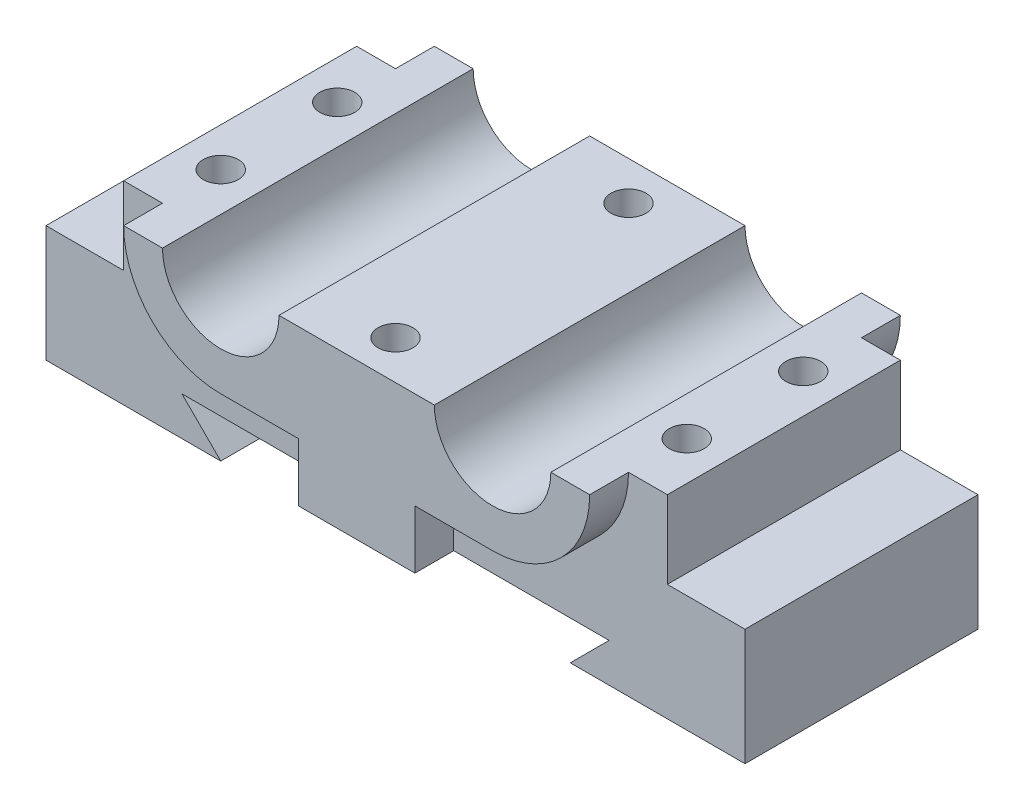
from build123d import *

# Parameters (mm, degrees)
BASE_BLOCK_DEPTH                 = 20
CENTER_POCKET_SKETCH_OUTSIDE_W   = 112.322
CENTER_POCKET_SKETCH_OUTSIDE_H   = 62.322
CENTER_POCKET_CUT_DEPTH          = 40
MOUNTING_HOLES_SKETCH_R          = 2.25
MOUNTING_HOLES_4_5_DEPTH         = 40
SADDLE_CUT_A_DEPTH               = 55
SADDLE_CUT_B_DEPTH               = 110
SADDLE_MIRROR_RIGHT_COPY_1_DEPTH = 110


with BuildPart() as part:
    # Base Profile Sketch → Base Block (new, symmetric)
    with BuildSketch(Plane.XY):
        Polygon((-35, 18.587360595), (-25, 18.587360595), (-10, 18.587360595), (10, 18.587360595), (25, 18.587360595), (35, 18.587360595), (35, 8.587360595), (45, 8.587360595), (45, -6.412639405), (22.5, -6.412639405), (27.5, -1.412639405), (-27.5, -1.412639405), (-22.5, -6.412639405), (-45, -6.412639405), (-45, 8.587360595), (-35, 8.587360595), align=None)
    extrude(amount=BASE_BLOCK_DEPTH, both=True)

    # Center Pocket Sketch outside → Center Pocket Cut (cut)
    with BuildSketch(Plane(origin=(0, 18.587360595, 0), x_dir=(1, 0, 0), z_dir=(0, 1, 0))):
        Rectangle(CENTER_POCKET_SKETCH_OUTSIDE_W, CENTER_POCKET_SKETCH_OUTSIDE_H)
        Polygon((30, 20), (-30, 20), (-30, 15), (-45, 15), (-45, -15), (-30, -15), (-30, -20), (30, -20), (30, -15), (45, -15), (45, 15), (30, 15), align=None, mode=Mode.SUBTRACT)
    extrude(amount=-CENTER_POCKET_CUT_DEPTH, mode=Mode.SUBTRACT)

    # Mounting Holes Sketch → Mounting Holes _4.5 (cut)
    with BuildSketch(Plane(origin=(0, 18.587360595, 0), x_dir=(1, 0, 0), z_dir=(0, 1, 0))):
        with Locations(Location((-30, 7.5, 0), (0, 0, 270))):
            Circle(MOUNTING_HOLES_SKETCH_R)
        with Locations(Location((-30, -7.5, 0), (0, 0, 180))):
            Circle(MOUNTING_HOLES_SKETCH_R)
        with Locations(Location((30, -7.5, 0), (0, 0, 270))):
            Circle(MOUNTING_HOLES_SKETCH_R)
        with Locations(Location((30, 7.5, 0), (0, 0, 180))):
            Circle(MOUNTING_HOLES_SKETCH_R)
        with Locations(Location((0, 15, 0), (0, 0, 270))):
            Circle(MOUNTING_HOLES_SKETCH_R)
        with Locations(Location((0, -15, 0), (0, 0, 180))):
            Circle(MOUNTING_HOLES_SKETCH_R)
    extrude(amount=-MOUNTING_HOLES_4_5_DEPTH, mode=Mode.SUBTRACT)

    # Saddle Profile Sketch → Saddle Cut A (cut, symmetric)
    with BuildSketch(Plane.XY.offset(15)):
        with BuildLine():
            Line((-10, 18.587360595), (-25, 18.587360595))
            ThreePointArc((-25, 18.587360595), (-17.5, 11.087360595), (-10, 18.587360595))
        make_face()
    saddle_cut_a = extrude(amount=SADDLE_CUT_A_DEPTH, both=True, mode=Mode.SUBTRACT)

    # Sketch5_7 → Saddle Cut B (cut)
    with BuildSketch(Plane.XY.offset(15)):
        with BuildLine():
            ThreePointArc((-17.5, 6.087360595), (-26.338834765, 9.74852583), (-30, 18.587360595))
            Line((-30, 18.587360595), (-30, -6.412639405))
            Line((-30, -6.412639405), (-22.5, -6.412639405))
            Line((-22.5, -6.412639405), (-27.5, -1.412639405))
            Line((-27.5, -1.412639405), (-7.5, -1.412639405))
            Line((-7.5, -1.412639405), (-7.5, 6.087360595))
            Line((-7.5, 6.087360595), (-17.5, 6.087360595))
        make_face()
    saddle_cut_b = extrude(amount=SADDLE_CUT_B_DEPTH, mode=Mode.SUBTRACT)

    # Saddle Mirror Front: Saddle Cut B across plane
    add(saddle_cut_b.mirror(Plane.XY), mode=Mode.SUBTRACT)

    # Saddle Mirror Right: Saddle Cut A, Saddle Cut B across plane
    add(saddle_cut_a.mirror(Plane(origin=(0, 0, 0), x_dir=(0, 0, 1), z_dir=(1, 0, 0))), mode=Mode.SUBTRACT)
    add(saddle_cut_b.mirror(Plane(origin=(0, 0, 0), x_dir=(0, 0, 1), z_dir=(1, 0, 0))), mode=Mode.SUBTRACT)

    # Saddle Mirror Right copy 1 sketch → Saddle Mirror Right copy 1 (cut)
    with BuildSketch(Plane(origin=(0, 0, -15), x_dir=(-1, 0, 0), z_dir=(0, 0, -1))):
        with BuildLine():
            ThreePointArc((-17.5, 6.087360595), (-26.338834765, 9.74852583), (-30, 18.587360595))
            Line((-30, 18.587360595), (-30, -6.412639405))
            Line((-30, -6.412639405), (-22.5, -6.412639405))
            Line((-22.5, -6.412639405), (-27.5, -1.412639405))
            Line((-27.5, -1.412639405), (-7.5, -1.412639405))
            Line((-7.5, -1.412639405), (-7.5, 6.087360595))
            Line((-7.5, 6.087360595), (-17.5, 6.087360595))
        make_face()
    extrude(amount=SADDLE_MIRROR_RIGHT_COPY_1_DEPTH, mode=Mode.SUBTRACT)


solid = part.part
